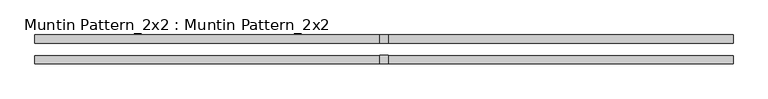
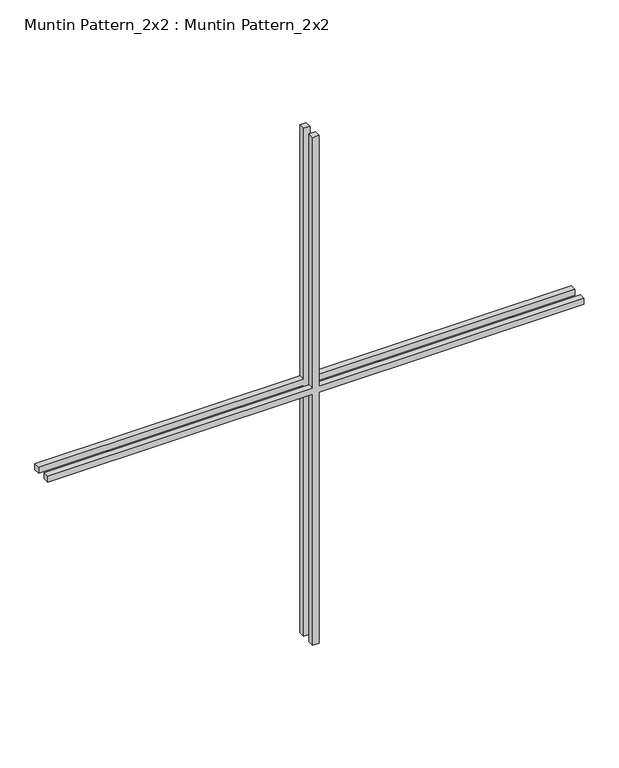
"""IFC4 building model written with IfcOpenShell, lengths in millimetres: proxy geometry, Muntin Pattern_2x2 : Muntin Pattern_2x2."""

from ifc_helpers import new_model, si_unit, frame, origin, place, context, project, spatial, polyline, outline, extrude, source, transform, mapped, element, save


def muntin_pattern_2x2_muntin_pattern_2x2_cef8da4c(model_context):
    return source(origin(), model_context, "Body", "SweptSolid", [
        extrude(outline(polyline([(546.1, -6.35), (546.1, -539.75), (533.4, -539.75), (533.4, -6.35), (0.0, -6.35), (0.0, 6.35), (533.4, 6.35), (533.4, 539.75), (546.1, 539.75), (546.1, 6.35), (1079.5, 6.35), (1079.5, -6.35), (546.1, -6.35)])), frame((0.0, -22.225, 0.0), z_axis=(0.0, 1.0, 0.0), x_axis=(0.0, 0.0, 1.0)), (0.0, 0.0, 1.0), 12.7),
        extrude(outline(polyline([(546.1, -6.35), (546.1, -539.75), (533.4, -539.75), (533.4, -6.35), (0.0, -6.35), (0.0, 6.35), (533.4, 6.35), (533.4, 539.75), (546.1, 539.75), (546.1, 6.35), (1079.5, 6.35), (1079.5, -6.35), (546.1, -6.35)])), frame((0.0, 9.525, 0.0), z_axis=(0.0, 1.0, 0.0), x_axis=(0.0, 0.0, 1.0)), (0.0, 0.0, 1.0), 12.7),
    ])


if __name__ == "__main__":
    model = new_model("IFC4")
    model_context = context("Model", 3, world=origin())
    ifc_project = project(units=[si_unit("LENGTHUNIT", "METRE", prefix="MILLI")], contexts=[model_context])
    site = spatial("IfcSite", under=ifc_project)
    building = spatial("IfcBuilding", under=site)
    placement = place(None, origin())
    muntin_pattern_2x2_muntin_pattern_2x2_shape = muntin_pattern_2x2_muntin_pattern_2x2_cef8da4c(model_context)
    element("IfcBuildingElementProxy", 1, Name="Muntin Pattern_2x2 : Muntin Pattern_2x2", ObjectType="Muntin Pattern_2x2 : Muntin Pattern_2x2", at=placement, inside=building, context=model_context, shape_type="MappedRepresentation", body=[
        mapped(muntin_pattern_2x2_muntin_pattern_2x2_shape, transform((0.0, 0.0, 0.0), x_axis=(1.0, 0.0, 0.0), y_axis=(0.0, 1.0, 0.0), z_axis=(0.0, 0.0, 1.0))),
    ])
    save(model, "model.ifc")

# Revit data of these elements
# Type "Muntin Pattern_2x2 : Muntin Pattern_2x2"
#   Width [instance default] = 4' - 0"
#   Thickness = 0' - 0 1/2"
#   Height [instance default] = 4' - 0"
#   Distance = 0' - 0 3/4"
#   Interior Material [instance default] = none
#   Exterior Material [instance default] = none
#   Default Elevation = 0
# Element 1 (IfcBuildingElementProxy, "Muntin Pattern_2x2 : Muntin Pattern_2x2")
#   Width = 3' - 6 1/2"
#   Height = 3' - 6 1/2"
#   Interior Material = Wood - Stained
#   Exterior Material = Clad - White
#   Materials on its faces: "Clad - White", "Wood - Stained"
# Materials
#   "Clad - White": class "Wood", colour RGB 242 242 238, transparency 0, Cost = 0
#   "Wood - Stained": class "Wood", colour RGB 224 178 126, transparency 0, Cost = 0
